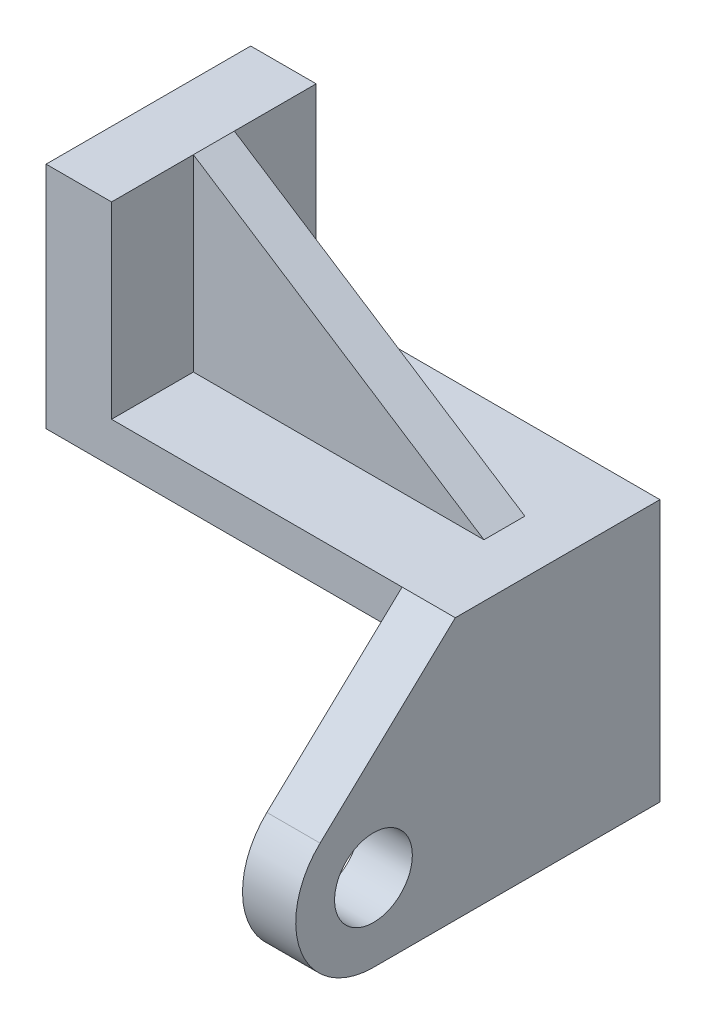
ISO-10303-21;
HEADER;
FILE_DESCRIPTION(('STEP AP214'),'2;1');
FILE_NAME('part.step','',(''),(''),'','','');
FILE_SCHEMA(('AUTOMOTIVE_DESIGN { 1 0 10303 214 1 1 1 1 }'));
ENDSEC;
DATA;
#1=APPLICATION_CONTEXT('core data for automotive mechanical design processes');
#2=APPLICATION_PROTOCOL_DEFINITION('international standard','automotive_design',2000,#1);
#3=PRODUCT_CONTEXT('',#1,'mechanical');
#4=PRODUCT('Part','Part','',(#3));
#5=PRODUCT_RELATED_PRODUCT_CATEGORY('part','',(#4));
#6=PRODUCT_DEFINITION_FORMATION('','',#4);
#7=PRODUCT_DEFINITION_CONTEXT('part definition',#1,'design');
#8=PRODUCT_DEFINITION('design','',#6,#7);
#9=PRODUCT_DEFINITION_SHAPE('','',#8);
#10=(LENGTH_UNIT() NAMED_UNIT(*) SI_UNIT(.MILLI.,.METRE.));
#11=(NAMED_UNIT(*) PLANE_ANGLE_UNIT() SI_UNIT($,.RADIAN.));
#12=(NAMED_UNIT(*) SI_UNIT($,.STERADIAN.) SOLID_ANGLE_UNIT());
#13=UNCERTAINTY_MEASURE_WITH_UNIT(LENGTH_MEASURE(1.E-05),#10,'distance_accuracy_value','');
#14=(GEOMETRIC_REPRESENTATION_CONTEXT(3) GLOBAL_UNCERTAINTY_ASSIGNED_CONTEXT((#13)) GLOBAL_UNIT_ASSIGNED_CONTEXT((#10,
#11,#12)) REPRESENTATION_CONTEXT('',''));
#15=CARTESIAN_POINT('',(0.,0.,0.));
#16=DIRECTION('',(0.,0.,1.));
#17=DIRECTION('',(1.,0.,0.));
#18=AXIS2_PLACEMENT_3D('',#15,#16,#17);
#19=CARTESIAN_POINT('',(87.,10.,20.));
#20=DIRECTION('',(0.543741302352791,0.839252879718438,0.));
#21=DIRECTION('',(-0.839252879718438,0.543741302352791,0.));
#22=AXIS2_PLACEMENT_3D('',#19,#20,#21);
#23=PLANE('',#22);
#24=DIRECTION('',(0.,0.,-1.));
#25=VECTOR('',#24,1.);
#26=CARTESIAN_POINT('',(16.,56.,50.));
#27=LINE('',#26,#25);
#28=CARTESIAN_POINT('',(16.,56.,30.));
#29=VERTEX_POINT('',#28);
#30=CARTESIAN_POINT('',(16.,56.,20.));
#31=VERTEX_POINT('',#30);
#32=EDGE_CURVE('E66',#29,#31,#27,.T.);
#33=ORIENTED_EDGE('',*,*,#32,.F.);
#34=DIRECTION('',(-0.839252879718438,0.543741302352791,0.));
#35=VECTOR('',#34,1.);
#36=CARTESIAN_POINT('',(87.,10.,30.));
#37=LINE('',#36,#35);
#38=CARTESIAN_POINT('',(87.,10.,30.));
#39=VERTEX_POINT('',#38);
#40=EDGE_CURVE('E145',#39,#29,#37,.T.);
#41=ORIENTED_EDGE('',*,*,#40,.F.);
#42=DIRECTION('',(0.,0.,1.));
#43=VECTOR('',#42,1.);
#44=CARTESIAN_POINT('',(87.,10.,20.));
#45=LINE('',#44,#43);
#46=CARTESIAN_POINT('',(87.,10.,20.));
#47=VERTEX_POINT('',#46);
#48=EDGE_CURVE('E231',#47,#39,#45,.T.);
#49=ORIENTED_EDGE('',*,*,#48,.F.);
#50=DIRECTION('',(-0.839252879718438,0.543741302352791,0.));
#51=VECTOR('',#50,1.);
#52=CARTESIAN_POINT('',(87.,10.,20.));
#53=LINE('',#52,#51);
#54=EDGE_CURVE('E155',#47,#31,#53,.T.);
#55=ORIENTED_EDGE('',*,*,#54,.T.);
#56=EDGE_LOOP('',(#33,#41,#49,#55));
#57=FACE_BOUND('',#56,.T.);
#58=ADVANCED_FACE('F44',(#57),#23,.T.);
#59=CARTESIAN_POINT('',(16.,56.,50.));
#60=DIRECTION('',(-1.,0.,0.));
#61=DIRECTION('',(0.,0.,1.));
#62=AXIS2_PLACEMENT_3D('',#59,#60,#61);
#63=PLANE('',#62);
#64=DIRECTION('',(0.,-1.,0.));
#65=VECTOR('',#64,1.);
#66=CARTESIAN_POINT('',(16.,56.,20.));
#67=LINE('',#66,#65);
#68=CARTESIAN_POINT('',(16.,10.,20.));
#69=VERTEX_POINT('',#68);
#70=EDGE_CURVE('E238',#31,#69,#67,.T.);
#71=ORIENTED_EDGE('',*,*,#70,.T.);
#72=DIRECTION('',(0.,0.,-1.));
#73=VECTOR('',#72,1.);
#74=CARTESIAN_POINT('',(16.,10.,50.));
#75=LINE('',#74,#73);
#76=CARTESIAN_POINT('',(16.,10.,0.));
#77=VERTEX_POINT('',#76);
#78=EDGE_CURVE('E159',#69,#77,#75,.T.);
#79=ORIENTED_EDGE('',*,*,#78,.T.);
#80=DIRECTION('',(0.,1.,0.));
#81=VECTOR('',#80,1.);
#82=CARTESIAN_POINT('',(16.,56.,0.));
#83=LINE('',#82,#81);
#84=CARTESIAN_POINT('',(16.,56.,0.));
#85=VERTEX_POINT('',#84);
#86=EDGE_CURVE('E180',#77,#85,#83,.T.);
#87=ORIENTED_EDGE('',*,*,#86,.T.);
#88=EDGE_CURVE('E152',#31,#85,#27,.T.);
#89=ORIENTED_EDGE('',*,*,#88,.F.);
#90=EDGE_LOOP('',(#71,#79,#87,#89));
#91=FACE_BOUND('',#90,.T.);
#92=ADVANCED_FACE('F257',(#91),#63,.F.);
#93=CARTESIAN_POINT('',(16.,0.,50.));
#94=DIRECTION('',(0.,1.,0.));
#95=DIRECTION('',(0.,0.,1.));
#96=AXIS2_PLACEMENT_3D('',#93,#94,#95);
#97=PLANE('',#96);
#98=DIRECTION('',(0.,0.,-1.));
#99=VECTOR('',#98,1.);
#100=CARTESIAN_POINT('',(87.,0.,50.));
#101=LINE('',#100,#99);
#102=CARTESIAN_POINT('',(87.,0.,50.));
#103=VERTEX_POINT('',#102);
#104=CARTESIAN_POINT('',(87.,0.,0.));
#105=VERTEX_POINT('',#104);
#106=EDGE_CURVE('E190',#103,#105,#101,.T.);
#107=ORIENTED_EDGE('',*,*,#106,.F.);
#108=DIRECTION('',(1.,0.,0.));
#109=VECTOR('',#108,1.);
#110=CARTESIAN_POINT('',(0.,0.,50.));
#111=LINE('',#110,#109);
#112=CARTESIAN_POINT('',(0.,0.,50.));
#113=VERTEX_POINT('',#112);
#114=EDGE_CURVE('E193',#113,#103,#111,.T.);
#115=ORIENTED_EDGE('',*,*,#114,.F.);
#116=DIRECTION('',(0.,0.,-1.));
#117=VECTOR('',#116,1.);
#118=CARTESIAN_POINT('',(0.,0.,50.));
#119=LINE('',#118,#117);
#120=CARTESIAN_POINT('',(0.,0.,0.));
#121=VERTEX_POINT('',#120);
#122=EDGE_CURVE('E11',#113,#121,#119,.T.);
#123=ORIENTED_EDGE('',*,*,#122,.T.);
#124=DIRECTION('',(1.,0.,0.));
#125=VECTOR('',#124,1.);
#126=CARTESIAN_POINT('',(16.,0.,0.));
#127=LINE('',#126,#125);
#128=EDGE_CURVE('E184',#121,#105,#127,.T.);
#129=ORIENTED_EDGE('',*,*,#128,.T.);
#130=EDGE_LOOP('',(#107,#115,#123,#129));
#131=FACE_BOUND('',#130,.T.);
#132=ADVANCED_FACE('F281',(#131),#97,.F.);
#133=CARTESIAN_POINT('',(0.,0.,50.));
#134=DIRECTION('',(0.,0.,-1.));
#135=DIRECTION('',(-1.,0.,0.));
#136=AXIS2_PLACEMENT_3D('',#133,#134,#135);
#137=PLANE('',#136);
#138=DIRECTION('',(0.,-1.,0.));
#139=VECTOR('',#138,1.);
#140=CARTESIAN_POINT('',(87.,0.,50.));
#141=LINE('',#140,#139);
#142=CARTESIAN_POINT('',(87.,10.,50.));
#143=VERTEX_POINT('',#142);
#144=EDGE_CURVE('E196',#143,#103,#141,.T.);
#145=ORIENTED_EDGE('',*,*,#144,.F.);
#146=DIRECTION('',(1.,0.,0.));
#147=VECTOR('',#146,1.);
#148=CARTESIAN_POINT('',(16.,10.,50.));
#149=LINE('',#148,#147);
#150=CARTESIAN_POINT('',(16.,10.,50.));
#151=VERTEX_POINT('',#150);
#152=EDGE_CURVE('E149',#151,#143,#149,.T.);
#153=ORIENTED_EDGE('',*,*,#152,.F.);
#154=DIRECTION('',(0.,-1.,0.));
#155=VECTOR('',#154,1.);
#156=CARTESIAN_POINT('',(16.,56.,50.));
#157=LINE('',#156,#155);
#158=CARTESIAN_POINT('',(16.,56.,50.));
#159=VERTEX_POINT('',#158);
#160=EDGE_CURVE('E248',#159,#151,#157,.T.);
#161=ORIENTED_EDGE('',*,*,#160,.F.);
#162=DIRECTION('',(-1.,0.,0.));
#163=VECTOR('',#162,1.);
#164=CARTESIAN_POINT('',(0.,56.,50.));
#165=LINE('',#164,#163);
#166=CARTESIAN_POINT('',(0.,56.,50.));
#167=VERTEX_POINT('',#166);
#168=EDGE_CURVE('E157',#159,#167,#165,.T.);
#169=ORIENTED_EDGE('',*,*,#168,.T.);
#170=DIRECTION('',(0.,-1.,0.));
#171=VECTOR('',#170,1.);
#172=CARTESIAN_POINT('',(0.,0.,50.));
#173=LINE('',#172,#171);
#174=EDGE_CURVE('E178',#167,#113,#173,.T.);
#175=ORIENTED_EDGE('',*,*,#174,.T.);
#176=ORIENTED_EDGE('',*,*,#114,.T.);
#177=EDGE_LOOP('',(#145,#153,#161,#169,#175,#176));
#178=FACE_BOUND('',#177,.T.);
#179=ADVANCED_FACE('F253',(#178),#137,.F.);
#180=CARTESIAN_POINT('',(0.,0.,50.));
#181=DIRECTION('',(1.,0.,0.));
#182=DIRECTION('',(0.,0.,-1.));
#183=AXIS2_PLACEMENT_3D('',#180,#181,#182);
#184=PLANE('',#183);
#185=DIRECTION('',(0.,-1.,0.));
#186=VECTOR('',#185,1.);
#187=CARTESIAN_POINT('',(0.,0.,0.));
#188=LINE('',#187,#186);
#189=CARTESIAN_POINT('',(0.,56.,0.));
#190=VERTEX_POINT('',#189);
#191=EDGE_CURVE('E187',#190,#121,#188,.T.);
#192=ORIENTED_EDGE('',*,*,#191,.T.);
#193=ORIENTED_EDGE('',*,*,#122,.F.);
#194=ORIENTED_EDGE('',*,*,#174,.F.);
#195=DIRECTION('',(0.,0.,-1.));
#196=VECTOR('',#195,1.);
#197=CARTESIAN_POINT('',(0.,56.,50.));
#198=LINE('',#197,#196);
#199=EDGE_CURVE('E162',#167,#190,#198,.T.);
#200=ORIENTED_EDGE('',*,*,#199,.T.);
#201=EDGE_LOOP('',(#192,#193,#194,#200));
#202=FACE_BOUND('',#201,.T.);
#203=ADVANCED_FACE('F50',(#202),#184,.F.);
#204=CARTESIAN_POINT('',(100.,0.,50.));
#205=DIRECTION('',(-1.,0.,0.));
#206=DIRECTION('',(0.,0.,1.));
#207=AXIS2_PLACEMENT_3D('',#204,#205,#206);
#208=PLANE('',#207);
#209=CARTESIAN_POINT('',(100.,-35.0000000000086,69.9999999999937));
#210=DIRECTION('',(1.,0.,0.));
#211=DIRECTION('',(0.,0.,-1.));
#212=AXIS2_PLACEMENT_3D('',#209,#210,#211);
#213=CIRCLE('',#212,9.49999999999941);
#214=CARTESIAN_POINT('',(100.,-35.0000000000086,60.4999999999943));
#215=VERTEX_POINT('',#214);
#216=EDGE_CURVE('E226',#215,#215,#213,.T.);
#217=ORIENTED_EDGE('',*,*,#216,.F.);
#218=EDGE_LOOP('',(#217));
#219=FACE_BOUND('',#218,.T.);
#220=DIRECTION('',(0.,0.,-1.));
#221=VECTOR('',#220,1.);
#222=CARTESIAN_POINT('',(100.,-54.0000000000076,0.));
#223=LINE('',#222,#221);
#224=CARTESIAN_POINT('',(100.,-54.0000000000081,69.9999999999937));
#225=VERTEX_POINT('',#224);
#226=CARTESIAN_POINT('',(100.,-54.0000000000076,0.));
#227=VERTEX_POINT('',#226);
#228=EDGE_CURVE('E216',#225,#227,#223,.T.);
#229=ORIENTED_EDGE('',*,*,#228,.T.);
#230=DIRECTION('',(0.,1.,0.));
#231=VECTOR('',#230,1.);
#232=CARTESIAN_POINT('',(100.,0.,0.));
#233=LINE('',#232,#231);
#234=CARTESIAN_POINT('',(100.,10.,0.));
#235=VERTEX_POINT('',#234);
#236=EDGE_CURVE('E185',#227,#235,#233,.T.);
#237=ORIENTED_EDGE('',*,*,#236,.T.);
#238=DIRECTION('',(0.,0.,-1.));
#239=VECTOR('',#238,1.);
#240=CARTESIAN_POINT('',(100.,10.,50.));
#241=LINE('',#240,#239);
#242=CARTESIAN_POINT('',(100.,10.,50.));
#243=VERTEX_POINT('',#242);
#244=EDGE_CURVE('E52',#243,#235,#241,.T.);
#245=ORIENTED_EDGE('',*,*,#244,.F.);
#246=DIRECTION('',(0.,-0.686353403912794,0.727268179516553));
#247=VECTOR('',#246,1.);
#248=CARTESIAN_POINT('',(100.,10.,50.));
#249=LINE('',#248,#247);
#250=CARTESIAN_POINT('',(100.,-21.1819045891944,83.0407146743365));
#251=VERTEX_POINT('',#250);
#252=EDGE_CURVE('E213',#243,#251,#249,.T.);
#253=ORIENTED_EDGE('',*,*,#252,.T.);
#254=CARTESIAN_POINT('',(100.,-35.0000000000086,69.9999999999937));
#255=DIRECTION('',(1.,0.,0.));
#256=DIRECTION('',(0.,0.,-1.));
#257=AXIS2_PLACEMENT_3D('',#254,#255,#256);
#258=CIRCLE('',#257,18.9999999999995);
#259=EDGE_CURVE('E207',#251,#225,#258,.T.);
#260=ORIENTED_EDGE('',*,*,#259,.T.);
#261=EDGE_LOOP('',(#229,#237,#245,#253,#260));
#262=FACE_BOUND('',#261,.T.);
#263=ADVANCED_FACE('F276',(#219,#262),#208,.F.);
#264=CARTESIAN_POINT('',(16.,10.,50.));
#265=DIRECTION('',(0.,-1.,0.));
#266=DIRECTION('',(0.,0.,-1.));
#267=AXIS2_PLACEMENT_3D('',#264,#265,#266);
#268=PLANE('',#267);
#269=DIRECTION('',(1.,0.,0.));
#270=VECTOR('',#269,1.);
#271=CARTESIAN_POINT('',(16.,10.,20.));
#272=LINE('',#271,#270);
#273=EDGE_CURVE('E240',#69,#47,#272,.T.);
#274=ORIENTED_EDGE('',*,*,#273,.T.);
#275=ORIENTED_EDGE('',*,*,#48,.T.);
#276=DIRECTION('',(1.,0.,0.));
#277=VECTOR('',#276,1.);
#278=CARTESIAN_POINT('',(16.,10.,30.));
#279=LINE('',#278,#277);
#280=CARTESIAN_POINT('',(16.,10.,30.));
#281=VERTEX_POINT('',#280);
#282=EDGE_CURVE('E58',#281,#39,#279,.T.);
#283=ORIENTED_EDGE('',*,*,#282,.F.);
#284=DIRECTION('',(0.,0.,1.));
#285=VECTOR('',#284,1.);
#286=CARTESIAN_POINT('',(16.,10.,30.));
#287=LINE('',#286,#285);
#288=EDGE_CURVE('E141',#281,#151,#287,.T.);
#289=ORIENTED_EDGE('',*,*,#288,.T.);
#290=ORIENTED_EDGE('',*,*,#152,.T.);
#291=DIRECTION('',(-1.,0.,0.));
#292=VECTOR('',#291,1.);
#293=CARTESIAN_POINT('',(16.,10.,50.));
#294=LINE('',#293,#292);
#295=EDGE_CURVE('E172',#243,#143,#294,.T.);
#296=ORIENTED_EDGE('',*,*,#295,.F.);
#297=ORIENTED_EDGE('',*,*,#244,.T.);
#298=DIRECTION('',(-1.,0.,0.));
#299=VECTOR('',#298,1.);
#300=CARTESIAN_POINT('',(16.,10.,0.));
#301=LINE('',#300,#299);
#302=EDGE_CURVE('E177',#235,#77,#301,.T.);
#303=ORIENTED_EDGE('',*,*,#302,.T.);
#304=ORIENTED_EDGE('',*,*,#78,.F.);
#305=EDGE_LOOP('',(#274,#275,#283,#289,#290,#296,#297,#303,#304));
#306=FACE_BOUND('',#305,.T.);
#307=ADVANCED_FACE('F251',(#306),#268,.F.);
#308=CARTESIAN_POINT('',(0.,56.,50.));
#309=DIRECTION('',(0.,-1.,0.));
#310=DIRECTION('',(0.,0.,-1.));
#311=AXIS2_PLACEMENT_3D('',#308,#309,#310);
#312=PLANE('',#311);
#313=DIRECTION('',(-1.,0.,0.));
#314=VECTOR('',#313,1.);
#315=CARTESIAN_POINT('',(0.,56.,0.));
#316=LINE('',#315,#314);
#317=EDGE_CURVE('E174',#85,#190,#316,.T.);
#318=ORIENTED_EDGE('',*,*,#317,.T.);
#319=ORIENTED_EDGE('',*,*,#199,.F.);
#320=ORIENTED_EDGE('',*,*,#168,.F.);
#321=EDGE_CURVE('E143',#159,#29,#27,.T.);
#322=ORIENTED_EDGE('',*,*,#321,.T.);
#323=ORIENTED_EDGE('',*,*,#32,.T.);
#324=ORIENTED_EDGE('',*,*,#88,.T.);
#325=EDGE_LOOP('',(#318,#319,#320,#322,#323,#324));
#326=FACE_BOUND('',#325,.T.);
#327=ADVANCED_FACE('F160',(#326),#312,.F.);
#328=CARTESIAN_POINT('',(0.,0.,0.));
#329=DIRECTION('',(0.,0.,-1.));
#330=DIRECTION('',(-1.,0.,0.));
#331=AXIS2_PLACEMENT_3D('',#328,#329,#330);
#332=PLANE('',#331);
#333=ORIENTED_EDGE('',*,*,#236,.F.);
#334=DIRECTION('',(1.,0.,0.));
#335=VECTOR('',#334,1.);
#336=CARTESIAN_POINT('',(87.,-54.0000000000076,0.));
#337=LINE('',#336,#335);
#338=CARTESIAN_POINT('',(87.,-54.0000000000076,0.));
#339=VERTEX_POINT('',#338);
#340=EDGE_CURVE('E205',#339,#227,#337,.T.);
#341=ORIENTED_EDGE('',*,*,#340,.F.);
#342=DIRECTION('',(0.,1.,0.));
#343=VECTOR('',#342,1.);
#344=CARTESIAN_POINT('',(87.,-54.0000000000076,0.));
#345=LINE('',#344,#343);
#346=EDGE_CURVE('E223',#339,#105,#345,.T.);
#347=ORIENTED_EDGE('',*,*,#346,.T.);
#348=ORIENTED_EDGE('',*,*,#128,.F.);
#349=ORIENTED_EDGE('',*,*,#191,.F.);
#350=ORIENTED_EDGE('',*,*,#317,.F.);
#351=ORIENTED_EDGE('',*,*,#86,.F.);
#352=ORIENTED_EDGE('',*,*,#302,.F.);
#353=EDGE_LOOP('',(#333,#341,#347,#348,#349,#350,#351,#352));
#354=FACE_BOUND('',#353,.T.);
#355=ADVANCED_FACE('F264',(#354),#332,.T.);
#356=CARTESIAN_POINT('',(87.,-35.0000000000086,69.9999999999937));
#357=DIRECTION('',(1.,0.,0.));
#358=DIRECTION('',(0.,0.,-1.));
#359=AXIS2_PLACEMENT_3D('',#356,#357,#358);
#360=PLANE('',#359);
#361=CARTESIAN_POINT('',(87.,-35.0000000000086,69.9999999999937));
#362=DIRECTION('',(1.,0.,0.));
#363=DIRECTION('',(0.,0.,-1.));
#364=AXIS2_PLACEMENT_3D('',#361,#362,#363);
#365=CIRCLE('',#364,9.49999999999941);
#366=CARTESIAN_POINT('',(87.,-35.0000000000086,60.4999999999943));
#367=VERTEX_POINT('',#366);
#368=EDGE_CURVE('E218',#367,#367,#365,.T.);
#369=ORIENTED_EDGE('',*,*,#368,.T.);
#370=EDGE_LOOP('',(#369));
#371=FACE_BOUND('',#370,.T.);
#372=ORIENTED_EDGE('',*,*,#144,.T.);
#373=ORIENTED_EDGE('',*,*,#106,.T.);
#374=ORIENTED_EDGE('',*,*,#346,.F.);
#375=DIRECTION('',(0.,0.,-1.));
#376=VECTOR('',#375,1.);
#377=CARTESIAN_POINT('',(87.,-54.0000000000076,0.));
#378=LINE('',#377,#376);
#379=CARTESIAN_POINT('',(87.,-54.0000000000081,69.9999999999937));
#380=VERTEX_POINT('',#379);
#381=EDGE_CURVE('E215',#380,#339,#378,.T.);
#382=ORIENTED_EDGE('',*,*,#381,.F.);
#383=CARTESIAN_POINT('',(87.,-35.0000000000086,69.9999999999937));
#384=DIRECTION('',(1.,0.,0.));
#385=DIRECTION('',(0.,0.,-1.));
#386=AXIS2_PLACEMENT_3D('',#383,#384,#385);
#387=CIRCLE('',#386,18.9999999999995);
#388=CARTESIAN_POINT('',(87.,-21.1819045891944,83.0407146743365));
#389=VERTEX_POINT('',#388);
#390=EDGE_CURVE('E206',#389,#380,#387,.T.);
#391=ORIENTED_EDGE('',*,*,#390,.F.);
#392=DIRECTION('',(0.,-0.686353403912794,0.727268179516553));
#393=VECTOR('',#392,1.);
#394=CARTESIAN_POINT('',(87.,10.,50.));
#395=LINE('',#394,#393);
#396=EDGE_CURVE('E225',#143,#389,#395,.T.);
#397=ORIENTED_EDGE('',*,*,#396,.F.);
#398=EDGE_LOOP('',(#372,#373,#374,#382,#391,#397));
#399=FACE_BOUND('',#398,.T.);
#400=ADVANCED_FACE('F269',(#371,#399),#360,.F.);
#401=CARTESIAN_POINT('',(87.,-54.0000000000076,0.));
#402=DIRECTION('',(0.,-1.,0.));
#403=DIRECTION('',(0.,0.,-1.));
#404=AXIS2_PLACEMENT_3D('',#401,#402,#403);
#405=PLANE('',#404);
#406=ORIENTED_EDGE('',*,*,#228,.F.);
#407=DIRECTION('',(1.,0.,0.));
#408=VECTOR('',#407,1.);
#409=CARTESIAN_POINT('',(87.,-54.0000000000081,69.9999999999937));
#410=LINE('',#409,#408);
#411=EDGE_CURVE('E203',#380,#225,#410,.T.);
#412=ORIENTED_EDGE('',*,*,#411,.F.);
#413=ORIENTED_EDGE('',*,*,#381,.T.);
#414=ORIENTED_EDGE('',*,*,#340,.T.);
#415=EDGE_LOOP('',(#406,#412,#413,#414));
#416=FACE_BOUND('',#415,.T.);
#417=ADVANCED_FACE('F284',(#416),#405,.T.);
#418=CARTESIAN_POINT('',(87.,-35.0000000000086,69.9999999999937));
#419=DIRECTION('',(1.,0.,0.));
#420=DIRECTION('',(0.,0.,-1.));
#421=AXIS2_PLACEMENT_3D('',#418,#419,#420);
#422=CYLINDRICAL_SURFACE('',#421,18.9999999999995);
#423=ORIENTED_EDGE('',*,*,#259,.F.);
#424=DIRECTION('',(1.,0.,0.));
#425=VECTOR('',#424,1.);
#426=CARTESIAN_POINT('',(87.,-21.1819045891944,83.0407146743365));
#427=LINE('',#426,#425);
#428=EDGE_CURVE('E202',#389,#251,#427,.T.);
#429=ORIENTED_EDGE('',*,*,#428,.F.);
#430=ORIENTED_EDGE('',*,*,#390,.T.);
#431=ORIENTED_EDGE('',*,*,#411,.T.);
#432=EDGE_LOOP('',(#423,#429,#430,#431));
#433=FACE_BOUND('',#432,.T.);
#434=ADVANCED_FACE('F282',(#433),#422,.T.);
#435=CARTESIAN_POINT('',(87.,10.,50.));
#436=DIRECTION('',(0.,0.727268179516553,0.686353403912794));
#437=DIRECTION('',(0.,-0.686353403912794,0.727268179516553));
#438=AXIS2_PLACEMENT_3D('',#435,#436,#437);
#439=PLANE('',#438);
#440=ORIENTED_EDGE('',*,*,#252,.F.);
#441=ORIENTED_EDGE('',*,*,#295,.T.);
#442=ORIENTED_EDGE('',*,*,#396,.T.);
#443=ORIENTED_EDGE('',*,*,#428,.T.);
#444=EDGE_LOOP('',(#440,#441,#442,#443));
#445=FACE_BOUND('',#444,.T.);
#446=ADVANCED_FACE('F277',(#445),#439,.T.);
#447=CARTESIAN_POINT('',(87.,-35.0000000000086,69.9999999999937));
#448=DIRECTION('',(1.,0.,0.));
#449=DIRECTION('',(0.,0.,-1.));
#450=AXIS2_PLACEMENT_3D('',#447,#448,#449);
#451=CYLINDRICAL_SURFACE('',#450,9.49999999999941);
#452=CARTESIAN_POINT('',(87.,-35.0000000000086,60.4999999999943));
#453=CARTESIAN_POINT('',(87.1354166666667,-35.0000000000086,60.4999999999943));
#454=CARTESIAN_POINT('',(87.2708333333333,-35.0000000000086,60.4999999999943));
#455=CARTESIAN_POINT('',(87.5416666666667,-35.0000000000086,60.4999999999943));
#456=CARTESIAN_POINT('',(87.6770833333333,-35.0000000000086,60.4999999999943));
#457=CARTESIAN_POINT('',(87.9479166666667,-35.0000000000086,60.4999999999943));
#458=CARTESIAN_POINT('',(88.0833333333333,-35.0000000000086,60.4999999999943));
#459=CARTESIAN_POINT('',(88.3541666666667,-35.0000000000086,60.4999999999943));
#460=CARTESIAN_POINT('',(88.4895833333333,-35.0000000000086,60.4999999999943));
#461=CARTESIAN_POINT('',(88.7604166666667,-35.0000000000086,60.4999999999943));
#462=CARTESIAN_POINT('',(88.8958333333333,-35.0000000000086,60.4999999999943));
#463=CARTESIAN_POINT('',(89.1666666666667,-35.0000000000086,60.4999999999943));
#464=CARTESIAN_POINT('',(89.3020833333333,-35.0000000000086,60.4999999999943));
#465=CARTESIAN_POINT('',(89.5729166666667,-35.0000000000086,60.4999999999943));
#466=CARTESIAN_POINT('',(89.7083333333333,-35.0000000000086,60.4999999999943));
#467=CARTESIAN_POINT('',(89.9791666666667,-35.0000000000086,60.4999999999943));
#468=CARTESIAN_POINT('',(90.1145833333333,-35.0000000000086,60.4999999999943));
#469=CARTESIAN_POINT('',(90.3854166666667,-35.0000000000086,60.4999999999943));
#470=CARTESIAN_POINT('',(90.5208333333333,-35.0000000000086,60.4999999999943));
#471=CARTESIAN_POINT('',(90.7916666666667,-35.0000000000086,60.4999999999943));
#472=CARTESIAN_POINT('',(90.9270833333333,-35.0000000000086,60.4999999999943));
#473=CARTESIAN_POINT('',(91.1979166666667,-35.0000000000086,60.4999999999943));
#474=CARTESIAN_POINT('',(91.3333333333333,-35.0000000000086,60.4999999999943));
#475=CARTESIAN_POINT('',(91.6041666666667,-35.0000000000086,60.4999999999943));
#476=CARTESIAN_POINT('',(91.7395833333333,-35.0000000000086,60.4999999999943));
#477=CARTESIAN_POINT('',(92.0104166666667,-35.0000000000086,60.4999999999943));
#478=CARTESIAN_POINT('',(92.1458333333333,-35.0000000000086,60.4999999999943));
#479=CARTESIAN_POINT('',(92.4166666666667,-35.0000000000086,60.4999999999943));
#480=CARTESIAN_POINT('',(92.5520833333333,-35.0000000000086,60.4999999999943));
#481=CARTESIAN_POINT('',(92.8229166666667,-35.0000000000086,60.4999999999943));
#482=CARTESIAN_POINT('',(92.9583333333333,-35.0000000000086,60.4999999999943));
#483=CARTESIAN_POINT('',(93.2291666666667,-35.0000000000086,60.4999999999943));
#484=CARTESIAN_POINT('',(93.3645833333333,-35.0000000000086,60.4999999999943));
#485=CARTESIAN_POINT('',(93.6354166666667,-35.0000000000086,60.4999999999943));
#486=CARTESIAN_POINT('',(93.7708333333333,-35.0000000000086,60.4999999999943));
#487=CARTESIAN_POINT('',(94.0416666666667,-35.0000000000086,60.4999999999943));
#488=CARTESIAN_POINT('',(94.1770833333333,-35.0000000000086,60.4999999999943));
#489=CARTESIAN_POINT('',(94.4479166666667,-35.0000000000086,60.4999999999943));
#490=CARTESIAN_POINT('',(94.5833333333333,-35.0000000000086,60.4999999999943));
#491=CARTESIAN_POINT('',(94.8541666666667,-35.0000000000086,60.4999999999943));
#492=CARTESIAN_POINT('',(94.9895833333333,-35.0000000000086,60.4999999999943));
#493=CARTESIAN_POINT('',(95.2604166666667,-35.0000000000086,60.4999999999943));
#494=CARTESIAN_POINT('',(95.3958333333333,-35.0000000000086,60.4999999999943));
#495=CARTESIAN_POINT('',(95.6666666666667,-35.0000000000086,60.4999999999943));
#496=CARTESIAN_POINT('',(95.8020833333333,-35.0000000000086,60.4999999999943));
#497=CARTESIAN_POINT('',(96.0729166666667,-35.0000000000086,60.4999999999943));
#498=CARTESIAN_POINT('',(96.2083333333333,-35.0000000000086,60.4999999999943));
#499=CARTESIAN_POINT('',(96.4791666666667,-35.0000000000086,60.4999999999943));
#500=CARTESIAN_POINT('',(96.6145833333333,-35.0000000000086,60.4999999999943));
#501=CARTESIAN_POINT('',(96.8854166666667,-35.0000000000086,60.4999999999943));
#502=CARTESIAN_POINT('',(97.0208333333333,-35.0000000000086,60.4999999999943));
#503=CARTESIAN_POINT('',(97.2916666666667,-35.0000000000086,60.4999999999943));
#504=CARTESIAN_POINT('',(97.4270833333333,-35.0000000000086,60.4999999999943));
#505=CARTESIAN_POINT('',(97.6979166666667,-35.0000000000086,60.4999999999943));
#506=CARTESIAN_POINT('',(97.8333333333333,-35.0000000000086,60.4999999999943));
#507=CARTESIAN_POINT('',(98.1041666666667,-35.0000000000086,60.4999999999943));
#508=CARTESIAN_POINT('',(98.2395833333333,-35.0000000000086,60.4999999999943));
#509=CARTESIAN_POINT('',(98.5104166666667,-35.0000000000086,60.4999999999943));
#510=CARTESIAN_POINT('',(98.6458333333333,-35.0000000000086,60.4999999999943));
#511=CARTESIAN_POINT('',(98.9166666666667,-35.0000000000086,60.4999999999943));
#512=CARTESIAN_POINT('',(99.0520833333333,-35.0000000000086,60.4999999999943));
#513=CARTESIAN_POINT('',(99.3229166666667,-35.0000000000086,60.4999999999943));
#514=CARTESIAN_POINT('',(99.4583333333333,-35.0000000000086,60.4999999999943));
#515=CARTESIAN_POINT('',(99.7291666666667,-35.0000000000086,60.4999999999943));
#516=CARTESIAN_POINT('',(99.8645833333333,-35.0000000000086,60.4999999999943));
#517=CARTESIAN_POINT('',(100.,-35.0000000000086,60.4999999999943));
#518=B_SPLINE_CURVE_WITH_KNOTS('',3,(#452,#453,#454,#455,#456,#457,#458,#459,#460,#461,#462,
#463,#464,#465,#466,#467,#468,#469,#470,#471,#472,#473,#474,#475,#476,#477,#478,#479,#480,#481,
#482,#483,#484,#485,#486,#487,#488,#489,#490,#491,#492,#493,#494,#495,#496,#497,#498,#499,#500,
#501,#502,#503,#504,#505,#506,#507,#508,#509,#510,#511,#512,#513,#514,#515,#516,#517),
.UNSPECIFIED.,.F.,.F.,(4,2,2,2,2,2,2,2,2,2,2,2,2,2,2,2,2,2,2,2,2,2,2,2,2,2,2,2,2,2,2,2,4),(0.,
0.406249999999997,0.812499999999994,1.21874999999999,1.62499999999999,2.03125,2.4375,
2.84374999999999,3.24999999999999,3.65624999999999,4.0625,4.46874999999999,4.87499999999999,
5.28124999999999,5.6875,6.09374999999999,6.49999999999999,6.90624999999999,7.31249999999999,
7.71875,8.12499999999999,8.53124999999999,8.93749999999999,9.34374999999998,9.74999999999999,
10.15625,10.5625,10.96875,11.375,11.78125,12.1875,12.59375,13.),.UNSPECIFIED.);
#519=EDGE_CURVE('BSEAM303',#367,#215,#518,.T.);
#520=ORIENTED_EDGE('',*,*,#368,.F.);
#521=ORIENTED_EDGE('',*,*,#216,.T.);
#522=ORIENTED_EDGE('',*,*,#519,.T.);
#523=ORIENTED_EDGE('',*,*,#519,.F.);
#524=EDGE_LOOP('',(#520,#522,#521,#523));
#525=FACE_BOUND('',#524,.T.);
#526=ADVANCED_FACE('F303',(#525),#451,.F.);
#527=CARTESIAN_POINT('',(0.,0.,20.));
#528=DIRECTION('',(0.,0.,1.));
#529=DIRECTION('',(1.,0.,0.));
#530=AXIS2_PLACEMENT_3D('',#527,#528,#529);
#531=PLANE('',#530);
#532=ORIENTED_EDGE('',*,*,#54,.F.);
#533=ORIENTED_EDGE('',*,*,#273,.F.);
#534=ORIENTED_EDGE('',*,*,#70,.F.);
#535=EDGE_LOOP('',(#532,#533,#534));
#536=FACE_BOUND('',#535,.T.);
#537=ADVANCED_FACE('F256',(#536),#531,.F.);
#538=CARTESIAN_POINT('',(16.,56.,30.));
#539=DIRECTION('',(-1.,0.,0.));
#540=DIRECTION('',(0.,0.,1.));
#541=AXIS2_PLACEMENT_3D('',#538,#539,#540);
#542=PLANE('',#541);
#543=ORIENTED_EDGE('',*,*,#160,.T.);
#544=ORIENTED_EDGE('',*,*,#288,.F.);
#545=DIRECTION('',(0.,-1.,0.));
#546=VECTOR('',#545,1.);
#547=CARTESIAN_POINT('',(16.,56.,30.));
#548=LINE('',#547,#546);
#549=EDGE_CURVE('E136',#29,#281,#548,.T.);
#550=ORIENTED_EDGE('',*,*,#549,.F.);
#551=ORIENTED_EDGE('',*,*,#321,.F.);
#552=EDGE_LOOP('',(#543,#544,#550,#551));
#553=FACE_BOUND('',#552,.T.);
#554=ADVANCED_FACE('F139',(#553),#542,.F.);
#555=CARTESIAN_POINT('',(0.,0.,30.));
#556=DIRECTION('',(0.,0.,1.));
#557=DIRECTION('',(1.,0.,0.));
#558=AXIS2_PLACEMENT_3D('',#555,#556,#557);
#559=PLANE('',#558);
#560=ORIENTED_EDGE('',*,*,#40,.T.);
#561=ORIENTED_EDGE('',*,*,#549,.T.);
#562=ORIENTED_EDGE('',*,*,#282,.T.);
#563=EDGE_LOOP('',(#560,#561,#562));
#564=FACE_BOUND('',#563,.T.);
#565=ADVANCED_FACE('F148',(#564),#559,.T.);
#566=CLOSED_SHELL('',(#58,#92,#132,#179,#203,#263,#307,#327,#355,#400,#417,#434,#446,#526,#537,
#554,#565));
#567=MANIFOLD_SOLID_BREP('B2',#566);
#568=ADVANCED_BREP_SHAPE_REPRESENTATION('',(#18,#567),#14);
#569=SHAPE_DEFINITION_REPRESENTATION(#9,#568);
ENDSEC;
END-ISO-10303-21;
